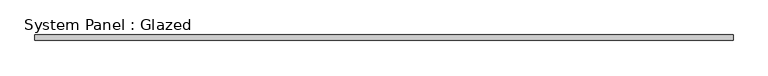
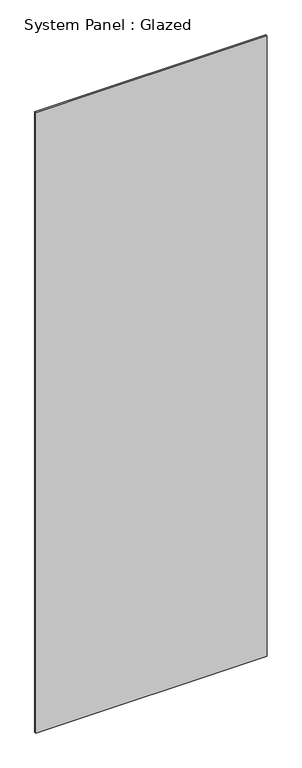
"""IFC4 building model written with IfcOpenShell, lengths in millimetres: plate geometry, System Panel : Glazed."""

from ifc_helpers import new_model, si_unit, origin, origin_with_axes, place, context, project, spatial, polyline, outline, extrude, source, transform, mapped, element, save


def system_panel_glazed_6b5749b4(model_context):
    return source(origin(), model_context, "Body", "SweptSolid", [
        extrude(outline(polyline([(1612.9, 19.05), (-1612.9, 19.05), (-1612.9, 44.45), (1612.9, 44.45), (1612.9, 19.05)])), origin_with_axes(), (0.0, 0.0, 1.0), 9144.0),
    ])


if __name__ == "__main__":
    model = new_model("IFC4")
    model_context = context("Model", 3, world=origin())
    ifc_project = project(units=[si_unit("LENGTHUNIT", "METRE", prefix="MILLI")], contexts=[model_context])
    site = spatial("IfcSite", under=ifc_project)
    building = spatial("IfcBuilding", under=site)
    placement = place(None, origin())
    system_panel_glazed_shape = system_panel_glazed_6b5749b4(model_context)
    element("IfcPlate", 1, ObjectType="System Panel : Glazed", at=placement, inside=building, context=model_context, shape_type="MappedRepresentation", body=[
        mapped(system_panel_glazed_shape, transform((0.0, 0.0, 0.0), x_axis=(1.0, 0.0, 0.0), y_axis=(0.0, 1.0, 0.0), z_axis=(0.0, 0.0, 1.0))),
    ])
    save(model, "model.ifc")

# Revit data of these elements
# Type "System Panel : Glazed"
#   Construction Type Id = "GSP4R"
#   Analytic Construction = "1/8 in Pilkington single glazing"
#   Visual Light Transmittance = 0.9
#   Solar Heat Gain Coefficient = 0.86
#   Heat Transfer Coefficient (U) = 1.18115 BTU/(h·ft²·°F)
#   Define Thermal Properties by = 1
# Element 1 (IfcPlate, "System Panel : Glazed")
#   Materials on its faces: "Glass"
# Materials
#   "Glass": class "Glass", colour RGB 0 128 192, transparency 0.75, Description = "Soda Lime Glass", Cost = 0
